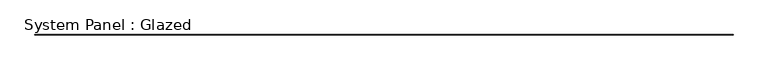
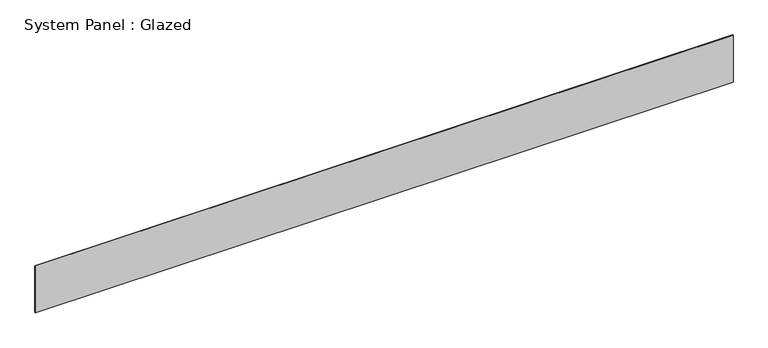
"""IFC4 building model written with IfcOpenShell, lengths in millimetres: plate geometry, System Panel : Glazed."""

from ifc_helpers import new_model, si_unit, origin, origin_with_axes, place, context, project, spatial, polyline, outline, extrude, source, transform, mapped, element, save


def system_panel_glazed_fd840cde(model_context):
    return source(origin(), model_context, "Body", "SweptSolid", [
        extrude(outline(polyline([(15773.4, 19.05), (-15773.4, 19.05), (-15773.4, 44.45), (15773.4, 44.45), (15773.4, 19.05)])), origin_with_axes(), (0.0, 0.0, 1.0), 2245.478727),
    ])


if __name__ == "__main__":
    model = new_model("IFC4")
    model_context = context("Model", 3, world=origin())
    ifc_project = project(units=[si_unit("LENGTHUNIT", "METRE", prefix="MILLI")], contexts=[model_context])
    site = spatial("IfcSite", under=ifc_project)
    building = spatial("IfcBuilding", under=site)
    placement = place(None, origin())
    system_panel_glazed_shape = system_panel_glazed_fd840cde(model_context)
    element("IfcPlate", 1, ObjectType="System Panel : Glazed", at=placement, inside=building, context=model_context, shape_type="MappedRepresentation", body=[
        mapped(system_panel_glazed_shape, transform((0.0, 0.0, 0.0), x_axis=(1.0, 0.0, 0.0), y_axis=(0.0, 1.0, 0.0), z_axis=(0.0, 0.0, 1.0))),
    ])
    save(model, "model.ifc")

# Revit data of these elements
# Type "System Panel : Glazed"
#   Construction Type Id = "GSP4R"
#   Analytic Construction = "1/8 in Pilkington single glazing"
#   Visual Light Transmittance = 0.9
#   Solar Heat Gain Coefficient = 0.86
#   Heat Transfer Coefficient (U) = 1.18115 BTU/(h·ft²·°F)
# Element 1 (IfcPlate, "System Panel : Glazed")
#   Materials on its faces: "Glass"
# Materials
#   "Glass": class "Glass", colour RGB 0 128 192, transparency 0.75, Description = "Soda Lime Glass", Cost = 0
